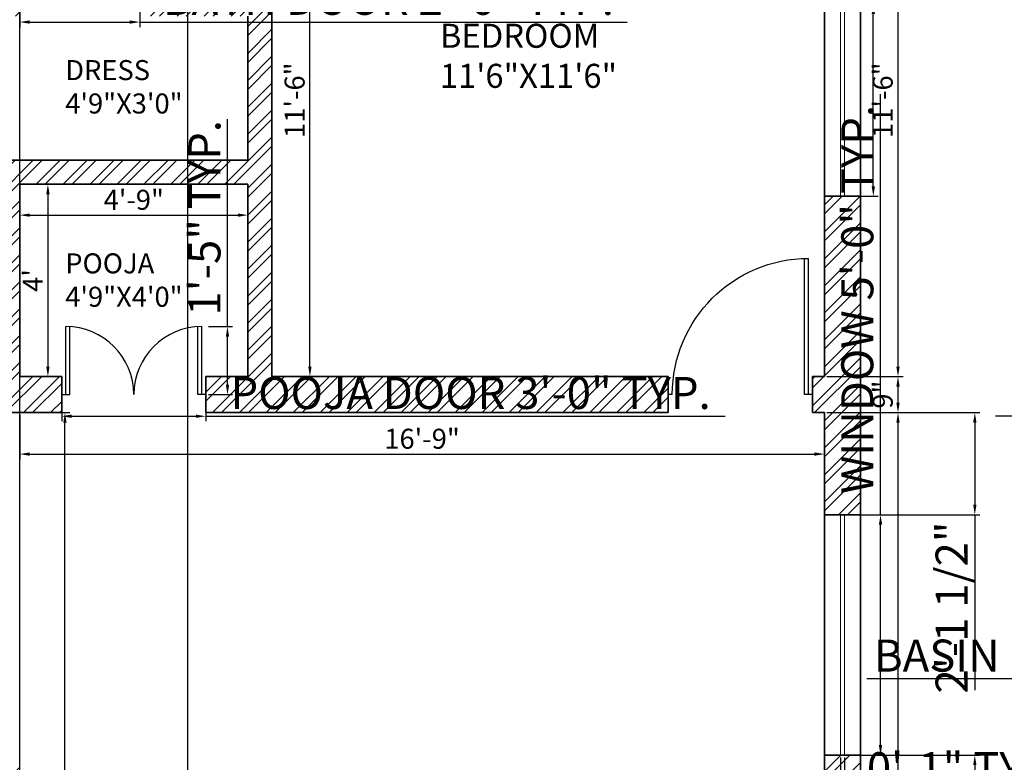
# Model space of a CAD drawing. Units: inches. Extents: x 3595 to 4516, y 2363 to 2965.
# Tile 4 of 12: x 3790 to 4036, y 2606 to 2791. Entities that reach past the tile are written whole.
import ezdxf

# ---------------------------------------------------------------- set-up
doc = ezdxf.new("R2010")
doc.units = ezdxf.units.IN
doc.linetypes.add('ACAD_ISO02W100', pattern=[15, 12, -3])
for name, color, linetype, lineweight in [('A-ANNO-DIMS', 2, 'Continuous', 18), ('A-AREA-IDEN', 7, 'Continuous', 18), ('A-DOOR', 4, 'Continuous', 25), ('A-GLAZ', 4, 'Continuous', 18), ('A-WALL', 7, 'Continuous', 35), ('A-WALL-OVHD', 7, 'ACAD_ISO02W100', 18)]:
    doc.layers.add(name, color=color, linetype=linetype, lineweight=lineweight)
doc.layers.add('A-WALL-PATT', color=251, linetype='Continuous', lineweight=13, true_color=0x636466)
doc.styles.get("Standard").update_dxf_attribs({"font": 'arial.ttf'})
doc.dimstyles.new('ISO-25', dxfattribs={"dimtxt": 8, "dimasz": 2.5, "dimexe": 1.25, "dimexo": 0.625, "dimtad": 1, "dimdec": 1, "dimlunit": 3, "dimtxsty": 'Standard', "dimcen": 2.5, "dimadec": 0, "dimazin": 0, "dimtfac": 1, "dimtdec": 1, "dimtmove": 0, "dimatfit": 3, "dimfxl": 1, "dimarcsym": 0})

# ---------------------------------------------------------------- blocks, each defined once
blk = doc.blocks.new('D1')
for p, q in [((1, 0), (1, 34)), ((2, 0), (2, 33.99)), ((0, 0), (2, 0)), ((35, 0), (36, 0))]:
    blk.add_line(p, q)
at = {"ltscale": 0.5}
blk.add_arc((1, 0), 34, 0, 90, dxfattribs=at)
blk = doc.blocks.new('D3')
for p, q in [((1, 0), (1, 17)), ((2, 0), (2, 16.97)), ((34, 0), (34, 16.97)), ((35, 0), (35, 17)), ((0, 0), (2, 0)), ((36, 0), (34, 0))]:
    blk.add_line(p, q)
at = {"ltscale": 0.5}
for centre, start, end in [((1, 0), 0, 90), ((35, 0), 90, 180)]:
    blk.add_arc(centre, 17, start, end, dxfattribs=at)
blk = doc.blocks.new('*D37')
at = {"layer": 'A-ANNO-DIMS', "color": 0, "lineweight": -2, "transparency": 16777216}
for p, q in [((3790.52, 2750.04), (3798.19, 2750.04)), ((3796.94, 2747.54), (3796.94, 2704.54)), ((3790.52, 2702.04), (3798.19, 2702.04))]:
    blk.add_line(p, q, dxfattribs=at)
at = {"layer": 'A-ANNO-DIMS', "color": 0, "transparency": 16777216}
for points in [[(3796.52, 2747.54), (3797.36, 2747.54), (3796.94, 2750.04)], [(3796.52, 2704.54), (3797.36, 2704.54), (3796.94, 2702.04)]]:
    blk.add_solid(points, dxfattribs=at)
at = {"layer": 'Defpoints', "color": 0, "transparency": 16777216}
for p in [(3789.89, 2750.04), (3789.89, 2702.04), (3796.94, 2702.04)]:
    blk.add_point(p, dxfattribs=at)
at = {"layer": 'A-ANNO-DIMS', "color": 0, "transparency": 16777216, "insert": (3793.81, 2726.04), "char_height": 5, "attachment_point": 5, "rotation": 90}
blk.add_mtext("4'", dxfattribs=at)
blk = doc.blocks.new('*D38')
at = {"layer": 'A-ANNO-DIMS', "color": 0, "lineweight": -2, "transparency": 16777216}
for p, q in [((3789.89, 2749.42), (3789.89, 2741.09)), ((3846.89, 2749.42), (3846.89, 2741.09)), ((3792.39, 2742.34), (3844.39, 2742.34))]:
    blk.add_line(p, q, dxfattribs=at)
at = {"layer": 'A-ANNO-DIMS', "color": 0, "transparency": 16777216}
for points in [[(3792.39, 2742.76), (3792.39, 2741.93), (3789.89, 2742.34)], [(3844.39, 2742.76), (3844.39, 2741.93), (3846.89, 2742.34)]]:
    blk.add_solid(points, dxfattribs=at)
at = {"layer": 'Defpoints', "color": 0, "transparency": 16777216}
for p in [(3789.89, 2750.04), (3846.89, 2750.04), (3846.89, 2742.34)]:
    blk.add_point(p, dxfattribs=at)
at = {"layer": 'A-ANNO-DIMS', "color": 0, "transparency": 16777216, "insert": (3818.39, 2745.52), "char_height": 5, "attachment_point": 5}
blk.add_mtext('4\'-9"', dxfattribs=at)
blk = doc.blocks.new('*D39')
at = {"layer": 'A-ANNO-DIMS', "color": 0, "lineweight": -2, "transparency": 16777216}
for p, q in [((3853.52, 2840.04), (3863.63, 2840.04)), ((3862.38, 2704.54), (3862.38, 2837.54)), ((3853.52, 2702.04), (3863.63, 2702.04))]:
    blk.add_line(p, q, dxfattribs=at)
at = {"layer": 'A-ANNO-DIMS', "color": 0, "transparency": 16777216}
for points in [[(3861.96, 2837.54), (3862.79, 2837.54), (3862.38, 2840.04)], [(3861.96, 2704.54), (3862.79, 2704.54), (3862.38, 2702.04)]]:
    blk.add_solid(points, dxfattribs=at)
at = {"layer": 'Defpoints', "color": 0, "transparency": 16777216}
for p in [(3852.89, 2840.04), (3862.38, 2840.04), (3852.89, 2702.04)]:
    blk.add_point(p, dxfattribs=at)
at = {"layer": 'A-ANNO-DIMS', "color": 0, "transparency": 16777216, "insert": (3859.2, 2771.04), "char_height": 5, "attachment_point": 5, "rotation": 90}
blk.add_mtext('11\'-6"', dxfattribs=at)
blk = doc.blocks.new('*D50')
at = {"layer": 'A-ANNO-DIMS', "color": 0, "lineweight": -2, "transparency": 16777216}
for p, q in [((3789.89, 2692.42), (3789.89, 2681.44)), ((3990.89, 2692.42), (3990.89, 2681.44)), ((3792.39, 2682.69), (3988.39, 2682.69))]:
    blk.add_line(p, q, dxfattribs=at)
at = {"layer": 'A-ANNO-DIMS', "color": 0, "transparency": 16777216}
for points in [[(3792.39, 2683.11), (3792.39, 2682.27), (3789.89, 2682.69)], [(3988.39, 2683.11), (3988.39, 2682.27), (3990.89, 2682.69)]]:
    blk.add_solid(points, dxfattribs=at)
at = {"layer": 'Defpoints', "color": 0, "transparency": 16777216}
for p in [(3789.89, 2693.04), (3990.89, 2693.04), (3990.89, 2682.69)]:
    blk.add_point(p, dxfattribs=at)
at = {"layer": 'A-ANNO-DIMS', "color": 0, "transparency": 16777216, "insert": (3890.39, 2685.87), "char_height": 5, "attachment_point": 5}
blk.add_mtext('16\'-9"', dxfattribs=at)
blk = doc.blocks.new('*D51')
at = {"layer": 'A-ANNO-DIMS', "color": 0, "lineweight": -2, "transparency": 16777216}
for p, q in [((3790.52, 2693.04), (3802.44, 2693.04)), ((3801.19, 2488.54), (3801.19, 2690.54)), ((3790.52, 2486.04), (3802.44, 2486.04))]:
    blk.add_line(p, q, dxfattribs=at)
at = {"layer": 'A-ANNO-DIMS', "color": 0, "transparency": 16777216}
for points in [[(3800.78, 2690.54), (3801.61, 2690.54), (3801.19, 2693.04)], [(3800.78, 2488.54), (3801.61, 2488.54), (3801.19, 2486.04)]]:
    blk.add_solid(points, dxfattribs=at)
at = {"layer": 'Defpoints', "color": 0, "transparency": 16777216}
for p in [(3789.89, 2693.04), (3801.19, 2693.04), (3789.89, 2486.04)]:
    blk.add_point(p, dxfattribs=at)
at = {"layer": 'A-ANNO-DIMS', "color": 0, "transparency": 16777216, "insert": (3798.01, 2589.54), "char_height": 5, "attachment_point": 5, "rotation": 90}
blk.add_mtext('17\'-3"', dxfattribs=at)
blk = doc.blocks.new('*D83')
at = {"layer": 'A-ANNO-DIMS', "color": 0, "lineweight": -2, "transparency": 16777216}
for p, q in [((3991.52, 2693.04), (4010.51, 2693.04)), ((4009.26, 2488.54), (4009.26, 2690.54)), ((3991.52, 2486.04), (4010.51, 2486.04))]:
    blk.add_line(p, q, dxfattribs=at)
at = {"layer": 'A-ANNO-DIMS', "color": 0, "transparency": 16777216}
for points in [[(4008.84, 2690.54), (4009.67, 2690.54), (4009.26, 2693.04)], [(4008.84, 2488.54), (4009.67, 2488.54), (4009.26, 2486.04)]]:
    blk.add_solid(points, dxfattribs=at)
at = {"layer": 'Defpoints', "color": 0, "transparency": 16777216}
for p in [(3990.89, 2693.04), (4009.26, 2693.04), (3990.89, 2486.04)]:
    blk.add_point(p, dxfattribs=at)
at = {"layer": 'A-ANNO-DIMS', "color": 0, "transparency": 16777216, "insert": (4006.08, 2589.54), "char_height": 5, "attachment_point": 5, "rotation": 90}
blk.add_mtext('17\'-3"', dxfattribs=at)
blk = doc.blocks.new('*D84')
at = {"layer": 'A-ANNO-DIMS', "color": 0, "lineweight": -2, "transparency": 16777216}
for p, q in [((3991.52, 2702.04), (4010.51, 2702.04)), ((4009.26, 2695.54), (4009.26, 2699.54)), ((3991.52, 2693.04), (4010.51, 2693.04))]:
    blk.add_line(p, q, dxfattribs=at)
at = {"layer": 'A-ANNO-DIMS', "color": 0, "transparency": 16777216}
for points in [[(4008.84, 2699.54), (4009.67, 2699.54), (4009.26, 2702.04)], [(4008.84, 2695.54), (4009.67, 2695.54), (4009.26, 2693.04)]]:
    blk.add_solid(points, dxfattribs=at)
at = {"layer": 'Defpoints', "color": 0, "transparency": 16777216}
for p in [(3990.89, 2702.04), (4009.26, 2702.04), (3990.89, 2693.04)]:
    blk.add_point(p, dxfattribs=at)
at = {"layer": 'A-ANNO-DIMS', "color": 0, "transparency": 16777216, "insert": (4006.08, 2697.54), "char_height": 5, "attachment_point": 5, "rotation": 90}
blk.add_mtext('9"', dxfattribs=at)
blk = doc.blocks.new('*D85')
at = {"layer": 'A-ANNO-DIMS', "color": 0, "lineweight": -2, "transparency": 16777216}
for p, q in [((3991.52, 2840.04), (4010.51, 2840.04)), ((4009.26, 2704.54), (4009.26, 2837.54)), ((3991.52, 2702.04), (4010.51, 2702.04))]:
    blk.add_line(p, q, dxfattribs=at)
at = {"layer": 'A-ANNO-DIMS', "color": 0, "transparency": 16777216}
for points in [[(4008.84, 2837.54), (4009.67, 2837.54), (4009.26, 2840.04)], [(4008.84, 2704.54), (4009.67, 2704.54), (4009.26, 2702.04)]]:
    blk.add_solid(points, dxfattribs=at)
at = {"layer": 'Defpoints', "color": 0, "transparency": 16777216}
for p in [(3990.89, 2840.04), (4009.26, 2840.04), (3990.89, 2702.04)]:
    blk.add_point(p, dxfattribs=at)
at = {"layer": 'A-ANNO-DIMS', "color": 0, "transparency": 16777216, "insert": (4006.08, 2771.04), "char_height": 5, "attachment_point": 5, "rotation": 90}
blk.add_mtext('11\'-6"', dxfattribs=at)
blk = doc.blocks.new('WIN-GLAZING-48IN')
for p, q in [((0, 1), (48, 1)), ((0, 0), (48, 0))]:
    blk.add_line(p, q)
blk = doc.blocks.new('WIN-GLAZING-60IN')
for p, q in [((0, 60), (0, 0)), ((1, 60), (1, 0))]:
    blk.add_line(p, q)
blk = doc.blocks.new('*D99')
at = {"layer": 'A-ANNO-DIMS', "color": 0, "lineweight": -2, "transparency": 16777216}
for p, q in [((4003.09, 2795.04), (4003.09, 2900.03)), ((3996.52, 2795.04), (4004.34, 2795.04)), ((4003.09, 2749.54), (4003.09, 2792.54)), ((3996.52, 2747.04), (4004.34, 2747.04))]:
    blk.add_line(p, q, dxfattribs=at)
at = {"layer": 'A-ANNO-DIMS', "color": 0, "transparency": 16777216}
for points in [[(4002.68, 2792.54), (4003.51, 2792.54), (4003.09, 2795.04)], [(4002.68, 2749.54), (4003.51, 2749.54), (4003.09, 2747.04)]]:
    blk.add_solid(points, dxfattribs=at)
at = {"layer": 'Defpoints', "color": 0, "transparency": 16777216}
for p in [(3995.89, 2795.04), (4003.09, 2795.04), (3995.89, 2747.04)]:
    blk.add_point(p, dxfattribs=at)
at = {"layer": 'A-ANNO-DIMS', "color": 0, "transparency": 16777216, "insert": (3998.33, 2848.79), "char_height": 8, "attachment_point": 5, "rotation": 90}
blk.add_mtext('WINDOW 4\'-0" TYP.', dxfattribs=at)
blk = doc.blocks.new('*D103')
at = {"layer": 'A-ANNO-DIMS', "color": 0, "lineweight": -2, "transparency": 16777216}
for p, q in [((4004.89, 2667.54), (4004.89, 2772.53)), ((3996.52, 2667.54), (4006.14, 2667.54)), ((4004.89, 2610.04), (4004.89, 2665.04)), ((3996.52, 2607.54), (4006.14, 2607.54))]:
    blk.add_line(p, q, dxfattribs=at)
at = {"layer": 'A-ANNO-DIMS', "color": 0, "transparency": 16777216}
for points in [[(4004.48, 2665.04), (4005.31, 2665.04), (4004.89, 2667.54)], [(4004.48, 2610.04), (4005.31, 2610.04), (4004.89, 2607.54)]]:
    blk.add_solid(points, dxfattribs=at)
at = {"layer": 'Defpoints', "color": 0, "transparency": 16777216}
for p in [(3995.89, 2667.54), (4004.89, 2667.54), (3995.89, 2607.54)]:
    blk.add_point(p, dxfattribs=at)
at = {"layer": 'A-ANNO-DIMS', "color": 0, "transparency": 16777216, "insert": (4000.13, 2721.29), "char_height": 8, "attachment_point": 5, "rotation": 90}
blk.add_mtext('WINDOW 5\'-0" TYP.', dxfattribs=at)
blk = doc.blocks.new('*D104')
at = {"layer": 'A-ANNO-DIMS', "color": 0, "lineweight": -2, "transparency": 16777216}
for p, q in [((3994.89, 2606.92), (3994.89, 2597.29)), ((3995.89, 2606.92), (3995.89, 2597.29)), ((3992.39, 2598.54), (3989.89, 2598.54)), ((3994.89, 2598.54), (3995.89, 2598.54)), ((3998.39, 2598.54), (4050.91, 2598.54))]:
    blk.add_line(p, q, dxfattribs=at)
at = {"layer": 'A-ANNO-DIMS', "color": 0, "transparency": 16777216}
for points in [[(3992.39, 2598.96), (3992.39, 2598.13), (3994.89, 2598.54)], [(3998.39, 2598.96), (3998.39, 2598.13), (3995.89, 2598.54)]]:
    blk.add_solid(points, dxfattribs=at)
at = {"layer": 'Defpoints', "color": 0, "transparency": 16777216}
for p in [(3994.89, 2607.54), (3995.89, 2607.54), (3995.89, 2598.54)]:
    blk.add_point(p, dxfattribs=at)
at = {"layer": 'A-ANNO-DIMS', "color": 0, "transparency": 16777216, "insert": (4025.9, 2603.25), "char_height": 8, "attachment_point": 5}
blk.add_mtext('0\'-1" TYP.', dxfattribs=at)
blk = doc.blocks.new('*D109')
at = {"layer": 'A-ANNO-DIMS', "color": 0, "lineweight": -2, "transparency": 16777216}
for p, q in [((3789.89, 2794.42), (3789.89, 2789.29)), ((3819.89, 2794.42), (3819.89, 2789.29)), ((3792.39, 2790.54), (3817.39, 2790.54)), ((3819.89, 2790.54), (3941.6, 2790.54))]:
    blk.add_line(p, q, dxfattribs=at)
at = {"layer": 'A-ANNO-DIMS', "color": 0, "transparency": 16777216}
for points in [[(3792.39, 2790.96), (3792.39, 2790.13), (3789.89, 2790.54)], [(3817.39, 2790.96), (3817.39, 2790.13), (3819.89, 2790.54)]]:
    blk.add_solid(points, dxfattribs=at)
at = {"layer": 'Defpoints', "color": 0, "transparency": 16777216}
for p in [(3789.89, 2795.04), (3819.89, 2795.04), (3819.89, 2790.54)]:
    blk.add_point(p, dxfattribs=at)
at = {"layer": 'A-ANNO-DIMS', "color": 0, "transparency": 16777216, "insert": (3881.99, 2795.31), "char_height": 8, "attachment_point": 5}
blk.add_mtext('BATH DOOR 2\'-6" TYP.', dxfattribs=at)
blk = doc.blocks.new('*D111')
at = {"layer": 'A-ANNO-DIMS', "color": 0, "lineweight": -2, "transparency": 16777216}
for p, q in [((3800.39, 2696.92), (3800.39, 2690.89)), ((3836.39, 2696.92), (3836.39, 2690.89)), ((3802.89, 2692.14), (3833.89, 2692.14)), ((3836.39, 2692.14), (3966.13, 2692.14))]:
    blk.add_line(p, q, dxfattribs=at)
at = {"layer": 'A-ANNO-DIMS', "color": 0, "transparency": 16777216}
for points in [[(3802.89, 2692.56), (3802.89, 2691.73), (3800.39, 2692.14)], [(3833.89, 2692.56), (3833.89, 2691.73), (3836.39, 2692.14)]]:
    blk.add_solid(points, dxfattribs=at)
at = {"layer": 'Defpoints', "color": 0, "transparency": 16777216}
for p in [(3800.39, 2697.54), (3836.39, 2697.54), (3836.39, 2692.14)]:
    blk.add_point(p, dxfattribs=at)
at = {"layer": 'A-ANNO-DIMS', "color": 0, "transparency": 16777216, "insert": (3902.51, 2696.91), "char_height": 8, "attachment_point": 5}
blk.add_mtext('POOJA DOOR 3\'-0" TYP.', dxfattribs=at)
blk = doc.blocks.new('*D112')
at = {"layer": 'A-ANNO-DIMS', "color": 0, "lineweight": -2, "transparency": 16777216}
for p, q in [((3841.79, 2714.54), (3841.79, 2766.3)), ((3837.02, 2714.54), (3843.04, 2714.54)), ((3841.79, 2700.04), (3841.79, 2712.04)), ((3837.02, 2697.54), (3843.04, 2697.54))]:
    blk.add_line(p, q, dxfattribs=at)
at = {"layer": 'A-ANNO-DIMS', "color": 0, "transparency": 16777216}
for points in [[(3841.38, 2712.04), (3842.21, 2712.04), (3841.79, 2714.54)], [(3841.38, 2700.04), (3842.21, 2700.04), (3841.79, 2697.54)]]:
    blk.add_solid(points, dxfattribs=at)
at = {"layer": 'Defpoints', "color": 0, "transparency": 16777216}
for p in [(3836.39, 2714.54), (3841.79, 2714.54), (3836.39, 2697.54)]:
    blk.add_point(p, dxfattribs=at)
at = {"layer": 'A-ANNO-DIMS', "color": 0, "transparency": 16777216, "insert": (3837.08, 2741.67), "char_height": 8, "attachment_point": 5, "rotation": 90}
blk.add_mtext('1\'-5" TYP.', dxfattribs=at)
blk = doc.blocks.new('*D115')
at = {"layer": 'A-ANNO-DIMS', "color": 0, "lineweight": -2, "transparency": 16777216}
for p, q in [((4183.24, 2696.92), (4183.24, 2690.89)), ((4219.24, 2696.92), (4219.24, 2690.89)), ((4183.24, 2692.14), (4033.6, 2692.14)), ((4216.74, 2692.14), (4185.74, 2692.14))]:
    blk.add_line(p, q, dxfattribs=at)
at = {"layer": 'A-ANNO-DIMS', "color": 0, "transparency": 16777216}
for points in [[(4185.74, 2692.56), (4185.74, 2691.73), (4183.24, 2692.14)], [(4216.74, 2692.56), (4216.74, 2691.73), (4219.24, 2692.14)]]:
    blk.add_solid(points, dxfattribs=at)
at = {"layer": 'Defpoints', "color": 0, "transparency": 16777216}
for p in [(4183.24, 2697.54), (4219.24, 2697.54), (4183.24, 2692.14)]:
    blk.add_point(p, dxfattribs=at)
at = {"layer": 'A-ANNO-DIMS', "color": 0, "transparency": 16777216, "insert": (4107.17, 2696.91), "char_height": 8, "attachment_point": 5}
blk.add_mtext('BEDROOM DOOR 3\'-0" TYP.', dxfattribs=at)
blk = doc.blocks.new('*D129')
at = {"layer": 'A-ANNO-DIMS', "color": 0, "lineweight": -2, "transparency": 16777216}
for p, q in [((4090.24, 2626.59), (4001.44, 2626.59)), ((4090.24, 2624.54), (4090.24, 2627.84)), ((4105.61, 2626.59), (4092.74, 2626.59)), ((4108.11, 2624.54), (4108.11, 2627.84))]:
    blk.add_line(p, q, dxfattribs=at)
at = {"layer": 'A-ANNO-DIMS', "color": 0, "transparency": 16777216}
for points in [[(4092.74, 2627.01), (4092.74, 2626.18), (4090.24, 2626.59)], [(4105.61, 2627.01), (4105.61, 2626.18), (4108.11, 2626.59)]]:
    blk.add_solid(points, dxfattribs=at)
at = {"layer": 'Defpoints', "color": 0, "transparency": 16777216}
for p in [(4090.24, 2626.59), (4090.24, 2623.91), (4108.11, 2623.91)]:
    blk.add_point(p, dxfattribs=at)
at = {"layer": 'A-ANNO-DIMS', "color": 0, "transparency": 16777216, "insert": (4044.59, 2631.35), "char_height": 8, "attachment_point": 5}
blk.add_mtext('BASIN 1\'-6" TYP.', dxfattribs=at)
blk = doc.blocks.new('*D154')
at = {"layer": 'A-ANNO-DIMS', "color": 0, "lineweight": -2, "transparency": 16777216}
for p, q in [((3991.52, 2693.04), (4029.69, 2693.04)), ((4028.44, 2690.54), (4028.44, 2670.04)), ((3991.52, 2667.54), (4029.69, 2667.54)), ((4028.44, 2667.54), (4028.44, 2623.75))]:
    blk.add_line(p, q, dxfattribs=at)
at = {"layer": 'A-ANNO-DIMS', "color": 0, "transparency": 16777216}
for points in [[(4028.03, 2690.54), (4028.86, 2690.54), (4028.44, 2693.04)], [(4028.03, 2670.04), (4028.86, 2670.04), (4028.44, 2667.54)]]:
    blk.add_solid(points, dxfattribs=at)
at = {"layer": 'Defpoints', "color": 0, "transparency": 16777216}
for p in [(3990.89, 2693.04), (3990.89, 2667.54), (4028.44, 2667.54)]:
    blk.add_point(p, dxfattribs=at)
at = {"layer": 'A-ANNO-DIMS', "color": 0, "transparency": 16777216, "insert": (4023.68, 2644.4), "char_height": 8, "attachment_point": 5, "rotation": 90}
blk.add_mtext('2\'-1 1/2"', dxfattribs=at)
blk = doc.blocks.new('*D155')
at = {"layer": 'A-ANNO-DIMS', "color": 0, "lineweight": -2, "transparency": 16777216}
for p, q in [((3991.52, 2607.54), (4029.69, 2607.54)), ((4028.44, 2605.04), (4028.44, 2574.04)), ((3991.52, 2571.54), (4029.69, 2571.54))]:
    blk.add_line(p, q, dxfattribs=at)
at = {"layer": 'A-ANNO-DIMS', "color": 0, "transparency": 16777216}
for points in [[(4028.03, 2605.04), (4028.86, 2605.04), (4028.44, 2607.54)], [(4028.03, 2574.04), (4028.86, 2574.04), (4028.44, 2571.54)]]:
    blk.add_solid(points, dxfattribs=at)
at = {"layer": 'Defpoints', "color": 0, "transparency": 16777216}
for p in [(3990.89, 2607.54), (3990.89, 2571.54), (4028.44, 2571.54)]:
    blk.add_point(p, dxfattribs=at)
at = {"layer": 'A-ANNO-DIMS', "color": 0, "transparency": 16777216, "insert": (4023.73, 2589.54), "char_height": 8, "attachment_point": 5, "rotation": 90}
blk.add_mtext('3\'-0"', dxfattribs=at)
blk = doc.blocks.new('*D157')
at = {"layer": 'A-ANNO-DIMS', "color": 0, "lineweight": -2, "transparency": 16777216}
for p, q in [((3789.89, 2486.67), (3789.89, 2932.84)), ((3792.39, 2931.59), (3829.39, 2931.59)), ((3831.89, 2486.67), (3831.89, 2932.84))]:
    blk.add_line(p, q, dxfattribs=at)
at = {"layer": 'A-ANNO-DIMS', "color": 0, "transparency": 16777216}
for points in [[(3792.39, 2932.01), (3792.39, 2931.18), (3789.89, 2931.59)], [(3829.39, 2932.01), (3829.39, 2931.18), (3831.89, 2931.59)]]:
    blk.add_solid(points, dxfattribs=at)
at = {"layer": 'Defpoints', "color": 0, "transparency": 16777216}
for p in [(3831.89, 2931.59), (3789.89, 2486.04), (3831.89, 2486.04)]:
    blk.add_point(p, dxfattribs=at)
at = {"layer": 'A-ANNO-DIMS', "color": 0, "transparency": 16777216, "insert": (3810.89, 2936.31), "char_height": 8, "attachment_point": 5}
blk.add_mtext('3\'-6"', dxfattribs=at)

msp = doc.modelspace()

# ---------------------------------------------------------------- hatches: boundary and pattern name
at = {"layer": 'A-WALL-PATT'}
h = msp.add_hatch(dxfattribs=at)
h.set_pattern_fill('ANSI32', color=256, scale=0.5)
h.paths.add_polyline_path([(3648.89, 2894.04), (3726.89, 2894.04), (3726.89, 2903.04), (3639.89, 2903.04), (3639.89, 2756.04), (3648.89, 2756.04)])
h.paths.add_polyline_path([(3800.39, 2903.04), (3774.89, 2903.04), (3774.89, 2894.04), (3780.89, 2894.04), (3780.89, 2792.04), (3789.89, 2792.04), (3789.89, 2894.04), (3800.39, 2894.04)])
h.paths.add_polyline_path([(3882.89, 2903.04), (3836.39, 2903.04), (3836.39, 2894.04), (3846.89, 2894.04), (3846.89, 2798.04), (3819.89, 2798.04), (3819.89, 2792.04), (3846.89, 2792.04), (3846.89, 2756.04), (3780.89, 2756.04), (3780.89, 2702.04), (3777.89, 2702.04), (3777.89, 2693.04), (3800.39, 2693.04), (3800.39, 2702.04), (3789.89, 2702.04), (3789.89, 2750.04), (3846.89, 2750.04), (3846.89, 2702.04), (3836.39, 2702.04), (3836.39, 2693.04), (3951.89, 2693.04), (3951.89, 2702.04), (3852.89, 2702.04), (3852.89, 2840.04), (3954.89, 2840.04), (3954.89, 2846.04), (3852.89, 2846.04), (3852.89, 2894.04), (3882.89, 2894.04)])
h.paths.add_polyline_path([(3999.89, 2903.04), (3918.89, 2903.04), (3918.89, 2894.04), (3948.89, 2894.04), (3948.89, 2876.04), (3954.89, 2876.04), (3954.89, 2894.04), (3990.89, 2894.04), (3990.89, 2795.04), (3999.89, 2795.04)])
h.paths.add_polyline_path([(3741.89, 2702.04), (3648.89, 2702.04), (3648.89, 2708.04), (3639.89, 2708.04), (3639.89, 2673.54), (3648.89, 2673.54), (3648.89, 2693.04), (3741.89, 2693.04)])
h.paths.add_polyline_path([(3648.89, 2600.04), (3741.89, 2600.04), (3741.89, 2606.04), (3648.89, 2606.04), (3648.89, 2625.54), (3639.89, 2625.54), (3639.89, 2561.04), (3648.89, 2561.04)])
h.paths.add_polyline_path([(3648.89, 2525.04), (3639.89, 2525.04), (3639.89, 2399.04), (3789.89, 2399.04), (3789.89, 2405.04), (3648.89, 2405.04), (3648.89, 2477.04), (3738.89, 2477.04), (3738.89, 2486.04), (3648.89, 2486.04)])
h.paths.add_polyline_path([(3789.89, 2606.04), (3777.89, 2606.04), (3777.89, 2600.04), (3780.89, 2600.04), (3780.89, 2486.04), (3774.89, 2486.04), (3774.89, 2477.04), (3831.89, 2477.04), (3831.89, 2486.04), (3789.89, 2486.04)])
h.paths.add_polyline_path([(3939.89, 2486.04), (3897.89, 2486.04), (3897.89, 2477.04), (3939.89, 2477.04)])
h.paths.add_polyline_path([(3999.89, 2511.54), (3990.89, 2511.54), (3990.89, 2486.04), (3987.89, 2486.04), (3987.89, 2477.04), (3999.89, 2477.04)])
h.paths.add_polyline_path([(3999.89, 2607.54), (3990.89, 2607.54), (3990.89, 2571.54), (3999.89, 2571.54)])
h.paths.add_polyline_path([(3999.89, 2747.04), (3990.89, 2747.04), (3990.89, 2702.04), (3987.89, 2702.04), (3987.89, 2693.04), (3990.89, 2693.04), (3990.89, 2667.54), (3999.89, 2667.54)])

# ---------------------------------------------------------------- linework, layer by layer
at = {"layer": 'A-WALL'}
for p, q in [((3990.89, 2894.04), (3990.89, 2702.04)), ((3852.89, 2840.04), (3852.89, 2702.04)), ((3846.89, 2756.04), (3846.89, 2792.04)), ((3780.89, 2756.04), (3846.89, 2756.04)), ((3789.89, 2750.04), (3846.89, 2750.04)), ((3789.89, 2702.04), (3789.89, 2750.04)), ((3846.89, 2702.04), (3846.89, 2750.04)), ((3990.89, 2747.04), (3999.89, 2747.04)), ((3789.89, 2702.04), (3800.39, 2702.04)), ((3800.39, 2702.04), (3800.39, 2693.04)), ((3836.39, 2702.04), (3836.39, 2693.04)), ((3836.39, 2702.04), (3846.89, 2702.04)), ((3852.89, 2702.04), (3951.89, 2702.04)), ((3951.89, 2702.04), (3951.89, 2693.04)), ((3987.89, 2702.04), (3987.89, 2693.04)), ((3987.89, 2702.04), (3990.89, 2702.04)), ((3777.89, 2693.04), (3800.39, 2693.04)), ((3836.39, 2693.04), (3951.89, 2693.04)), ((3987.89, 2693.04), (3990.89, 2693.04)), ((3990.89, 2693.04), (3990.89, 2486.04)), ((3999.89, 2667.54), (3990.89, 2667.54)), ((3999.89, 2607.54), (3990.89, 2607.54))]:
    msp.add_line(p, q, dxfattribs=at)
msp.add_lwpolyline([(3789.89, 2399.04), (3639.89, 2399.04), (3639.89, 2903.04), (3999.89, 2903.04), (3999.89, 2477.04)], dxfattribs=at)
at = {"layer": 'A-WALL-OVHD', "ltscale": 0.5}
msp.add_line((3789.89, 2606.04), (3789.89, 2693.04), dxfattribs=at)

# ---------------------------------------------------------------- block references
at = {"layer": 'A-DOOR', "xscale": -1}
msp.add_blockref('D1', (3987.89, 2697.54), dxfattribs=at)
at = {"layer": 'A-DOOR'}
msp.add_blockref('D3', (3800.39, 2697.54), dxfattribs=at)
at = {"layer": 'A-GLAZ', "rotation": 90.00000000000108}
msp.add_blockref('WIN-GLAZING-48IN', (3995.89, 2747.04), dxfattribs=at)
at = {"layer": 'A-GLAZ'}
msp.add_blockref('WIN-GLAZING-60IN', (3994.89, 2607.54), dxfattribs=at)

# ---------------------------------------------------------------- texts
at = {"layer": 'A-AREA-IDEN', "attachment_point": 1}
for s, insert, char_height in [('{\\fTimes New Roman|b0|i0|c0|p18;BEDROOM\\P11\'6"X11\'6"}', (3894.84, 2790.12), 6), ('{\\fTimes New Roman|b0|i0|c0|p18;DRESS\\P4\'9"X3\'0"}', (3801.27, 2781.05), 5), ('{\\fTimes New Roman|b0|i0|c0|p18;POOJA\\P4\'9"X4\'0"}', (3801.27, 2732.8), 5)]:
    msp.add_mtext_dynamic_manual_height_columns(s, width=67.3508, gutter_width=12.5, heights=[0], dxfattribs=dict(at, insert=insert, char_height=char_height))

# ---------------------------------------------------------------- dimensions: what is measured, and where the dimension line sits
at = {"layer": 'A-ANNO-DIMS'}
for base, p1, p2, override, picture, middle in [((3831.89, 2931.59), (3789.89, 2486.04), (3831.89, 2486.04), {"dimdec": 1, "dimlfac": 1, "dimrnd": 0, "dimzin": 1, "dimdsep": 46, "dimlunit": 4, "dimfrac": 2}, '*D157', (3810.89, 2936.31)), ((3846.89, 2742.34), (3789.89, 2750.04), (3846.89, 2750.04), {"dimtxt": 5, "dimclrd": 0, "dimclre": 0, "dimclrt": 0}, '*D38', (3818.39, 2745.52)), ((3990.89, 2682.69), (3789.89, 2693.04), (3990.89, 2693.04), {"dimtxt": 5, "dimclrd": 0, "dimclre": 0, "dimclrt": 0}, '*D50', (3890.39, 2685.87))]:
    dim = msp.add_linear_dim(base=base, p1=p1, p2=p2, dimstyle='ISO-25', override=override, dxfattribs=at)
    dim.commit()
    dim.dimension.update_dxf_attribs({"geometry": picture, "text_midpoint": middle})
for base, p1, p2, angle, text, picture, middle in [((4003.09, 2795.04), (3995.89, 2747.04), (3995.89, 2795.04), 90, 'WINDOW <> TYP.', '*D99', (3998.33, 2848.79)), ((4004.89, 2667.54), (3995.89, 2607.54), (3995.89, 2667.54), 90, 'WINDOW <> TYP.', '*D103', (4000.13, 2721.29)), ((3841.79, 2714.54), (3836.39, 2697.54), (3836.39, 2714.54), 90, '<> TYP.', '*D112', (3837.08, 2741.67)), ((4183.24, 2692.14), (4219.24, 2697.54), (4183.24, 2697.54), 180, 'BEDROOM DOOR <> TYP.', '*D115', (4107.17, 2696.91)), ((4090.24, 2626.59), (4108.11, 2623.91), (4090.24, 2623.91), 180, 'BASIN <> TYP.', '*D129', (4044.59, 2631.35))]:
    dim = msp.add_linear_dim(base=base, p1=p1, p2=p2, angle=angle, text=text, dimstyle='ISO-25', override={"dimdec": 1, "dimlfac": 1, "dimrnd": 0, "dimzin": 1, "dimdsep": 46, "dimlunit": 4, "dimfrac": 2}, dxfattribs=at)
    dim.commit()
    dim.dimension.update_dxf_attribs({"geometry": picture, "text_midpoint": middle})
for base, p1, p2, override, picture, middle in [((3862.38, 2840.04), (3852.89, 2702.04), (3852.89, 2840.04), {"dimtxt": 5, "dimclrd": 0, "dimclre": 0, "dimclrt": 0}, '*D39', (3859.2, 2771.04)), ((4009.26, 2840.04), (3990.89, 2702.04), (3990.89, 2840.04), {"dimtxt": 5, "dimclrd": 0, "dimclre": 0, "dimclrt": 0, "dimtmove": 1}, '*D85', (4006.08, 2771.04)), ((3796.94, 2702.04), (3789.89, 2750.04), (3789.89, 2702.04), {"dimtxt": 5, "dimclrd": 0, "dimclre": 0, "dimclrt": 0}, '*D37', (3793.81, 2726.04)), ((4009.26, 2702.04), (3990.89, 2693.04), (3990.89, 2702.04), {"dimtxt": 5, "dimclrd": 0, "dimclre": 0, "dimclrt": 0, "dimtmove": 1}, '*D84', (4006.08, 2697.54)), ((3801.19, 2693.04), (3789.89, 2486.04), (3789.89, 2693.04), {"dimtxt": 5, "dimclrd": 0, "dimclre": 0, "dimclrt": 0}, '*D51', (3798.01, 2589.54)), ((4009.26, 2693.04), (3990.89, 2486.04), (3990.89, 2693.04), {"dimtxt": 5, "dimclrd": 0, "dimclre": 0, "dimclrt": 0, "dimtmove": 1}, '*D83', (4006.08, 2589.54)), ((4028.44, 2667.54), (3990.89, 2693.04), (3990.89, 2667.54), {"dimdec": 1, "dimlfac": 1, "dimrnd": 0, "dimzin": 1, "dimdsep": 46, "dimlunit": 4, "dimfrac": 2}, '*D154', (4023.68, 2644.4)), ((4028.44, 2571.54), (3990.89, 2607.54), (3990.89, 2571.54), {"dimdec": 1, "dimlfac": 1, "dimrnd": 0, "dimzin": 1, "dimdsep": 46, "dimlunit": 4, "dimfrac": 2}, '*D155', (4023.73, 2589.54))]:
    dim = msp.add_linear_dim(base=base, p1=p1, p2=p2, angle=90, dimstyle='ISO-25', override=override, dxfattribs=at)
    dim.commit()
    dim.dimension.update_dxf_attribs({"geometry": picture, "text_midpoint": middle})
for base, p1, p2, text, picture, middle in [((3819.89, 2790.54), (3789.89, 2795.04), (3819.89, 2795.04), 'BATH DOOR <> TYP.', '*D109', (3881.99, 2795.31)), ((3836.39, 2692.14), (3800.39, 2697.54), (3836.39, 2697.54), 'POOJA DOOR <> TYP.', '*D111', (3902.51, 2696.91)), ((3995.89, 2598.54), (3994.89, 2607.54), (3995.89, 2607.54), '<> TYP.', '*D104', (4025.9, 2603.25))]:
    dim = msp.add_linear_dim(base=base, p1=p1, p2=p2, text=text, dimstyle='ISO-25', override={"dimdec": 1, "dimlfac": 1, "dimrnd": 0, "dimzin": 1, "dimdsep": 46, "dimlunit": 4, "dimfrac": 2}, dxfattribs=at)
    dim.commit()
    dim.dimension.update_dxf_attribs({"geometry": picture, "text_midpoint": middle})

doc.saveas('drawing.dxf')
